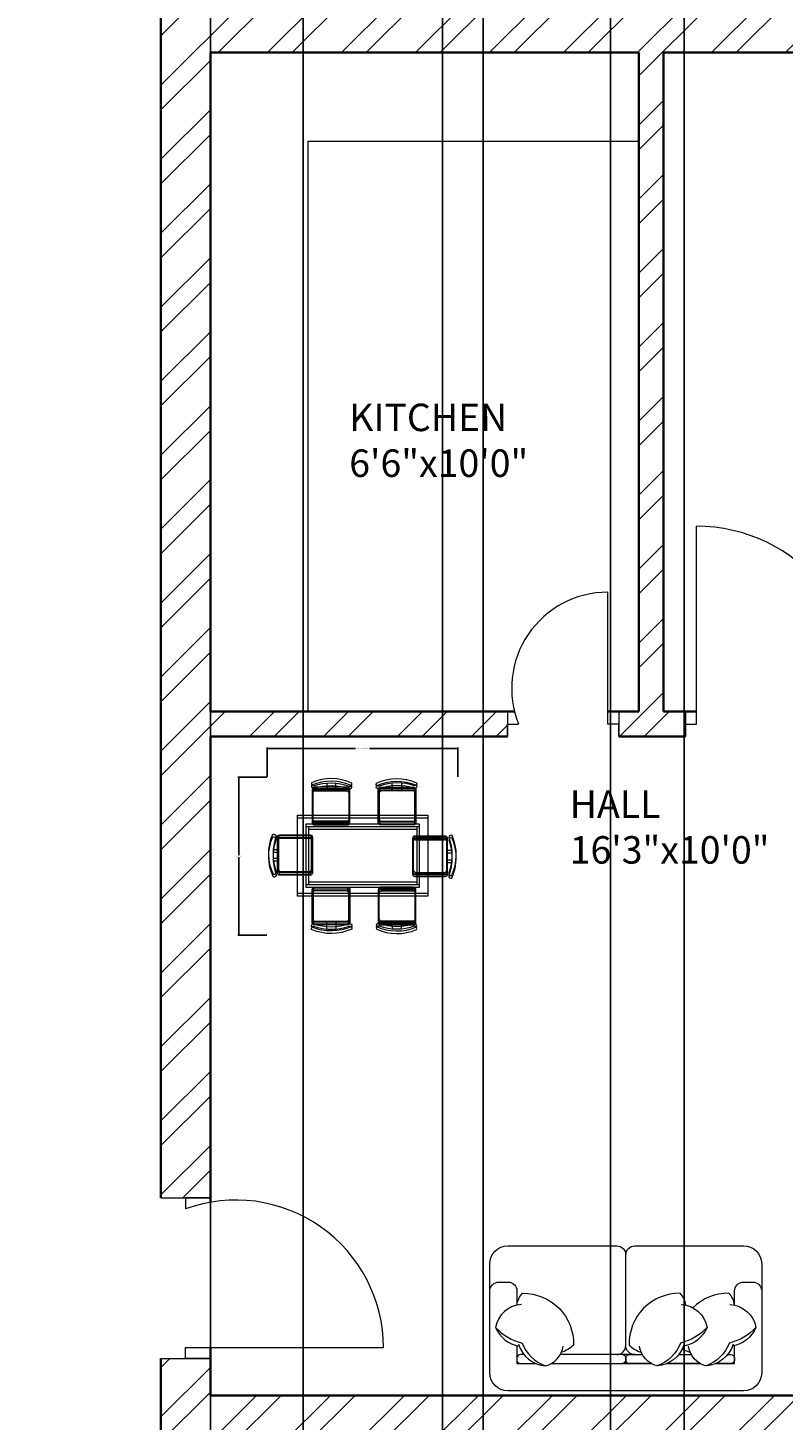
# Model space of a CAD drawing. Units: inches. Extents: x 2552 to 3217, y 1417 to 2737.
# Tile 12 of 25: x 2885 to 3022, y 1885 to 2138. Entities that reach past the tile are written whole.
import ezdxf

# ---------------------------------------------------------------- set-up
doc = ezdxf.new("R2010")
doc.units = ezdxf.units.IN
for name, color, linetype, lineweight in [('A-ANNO-DIMS', 2, 'Continuous', 18), ('A-AREA-IDEN', 7, 'Continuous', 18), ('A-DOOR', 21, 'Continuous', 18), ('A-FLOR-CASE', 9, 'Continuous', 18), ('A-FURN', 8, 'Continuous', 13), ('A-WALL', 7, 'Continuous', 35), ('A-WALL-PATT', 217, 'Continuous', 13)]:
    doc.layers.add(name, color=color, linetype=linetype, lineweight=lineweight)
doc.styles.get("Standard").update_dxf_attribs({"font": 'arial.ttf'})
doc.dimstyles.get("Standard").update_dxf_attribs({"dimtxt": 0.18, "dimasz": 0.18, "dimexe": 0.18, "dimexo": 0.0625, "dimgap": 0.09, "dimtad": 0, "dimtih": 1, "dimtoh": 1, "dimdec": 4, "dimzin": 0, "dimdsep": 46, "dimtxsty": 'Standard', "dimcen": 0.09, "dimadec": 0, "dimazin": 0, "dimtfac": 1, "dimtdec": 4, "dimtofl": 0, "dimtmove": 0, "dimatfit": 3, "dimfxl": 1, "dimtolj": 1, "dimtzin": 0, "dimarcsym": 0})

# ---------------------------------------------------------------- blocks, each defined once
blk = doc.blocks.new('DINING-SET-SIX')
for points in [[(8.15, 26.89, -0.175809), (14.62, 26.84, 0.578392), (15.11, 27.38, 0.214524), (7.8, 27.47, 0.552014), (8.15, 26.89, -0.065079)], [(8.15, 26.89, -0.175809), (14.62, 26.84, 0.578392), (15.11, 27.38, 0.214524), (7.8, 27.47, 0.552014), (8.15, 26.89, -0.065079)], [(20.07, 26.84, -0.578392), (19.58, 27.38, -0.214524), (26.89, 27.47, -0.552014), (26.55, 26.89, 0.175809), (20.07, 26.84)], [(20.07, 26.84, -0.578392), (19.58, 27.38, -0.214524), (26.89, 27.47, -0.552014), (26.55, 26.89, 0.175809), (20.07, 26.84)], [(8.15, 26.41, -0.175809), (14.62, 26.36, 0.578392), (15.11, 26.9, 0.214524), (7.8, 27, 0.552014), (8.15, 26.41, -0.065079)], [(8.15, 26.41, -0.175809), (14.62, 26.36, 0.578392), (15.11, 26.9, 0.214524), (7.8, 27, 0.552014), (8.15, 26.41, -0.065079)], [(14.35, 26.63), (8.33, 26.63, 0.414214), (7.91, 26.21), (7.91, 20.68, 0.414214), (8.33, 20.26), (14.35, 20.26, 0.414214), (14.77, 20.68), (14.77, 26.21, 0.414214), (14.35, 26.63)], [(14.35, 26.63), (8.33, 26.63, 0.414214), (7.91, 26.21), (7.91, 20.68, 0.414214), (8.33, 20.26), (14.35, 20.26, 0.414214), (14.77, 20.68), (14.77, 26.21, 0.414214), (14.35, 26.63)], [(14.35, 26.15), (8.33, 26.15, 0.414214), (7.91, 25.73), (7.91, 20.2, 0.414214), (8.33, 19.78), (14.35, 19.78, 0.414214), (14.77, 20.2), (14.77, 25.73, 0.414214), (14.35, 26.15)], [(14.35, 26.15), (8.33, 26.15, 0.414214), (7.91, 25.73), (7.91, 20.2, 0.414214), (8.33, 19.78), (14.35, 19.78, 0.414214), (14.77, 20.2), (14.77, 25.73, 0.414214), (14.35, 26.15)], [(12.23, 26.63), (12.23, 27.39, -0.064759)], [(12.23, 26.63), (12.23, 27.39, -0.064759)], [(12.23, 26.15), (12.23, 26.91, -0.064759)], [(12.23, 26.15), (12.23, 26.91, -0.064759)], [(20.07, 26.36, -0.578392), (19.58, 26.9, -0.214524), (26.89, 27, -0.552014), (26.55, 26.41, 0.175809), (20.07, 26.36)], [(20.07, 26.36, -0.578392), (19.58, 26.9, -0.214524), (26.89, 27, -0.552014), (26.55, 26.41, 0.175809), (20.07, 26.36)], [(26.36, 26.63, -0.414214), (26.78, 26.21), (26.78, 20.68, -0.414214), (26.36, 20.26), (20.35, 20.26, -0.414214), (19.92, 20.68), (19.92, 26.21, -0.414214), (20.35, 26.63), (26.36, 26.63)], [(26.36, 26.63, -0.414214), (26.78, 26.21), (26.78, 20.68, -0.414214), (26.36, 20.26), (20.35, 20.26, -0.414214), (19.92, 20.68), (19.92, 26.21, -0.414214), (20.35, 26.63), (26.36, 26.63)], [(26.36, 26.15, -0.414214), (26.78, 25.73), (26.78, 20.2, -0.414214), (26.36, 19.78), (20.35, 19.78, -0.414214), (19.92, 20.2), (19.92, 25.73, -0.414214), (20.35, 26.15), (26.36, 26.15)], [(26.36, 26.15, -0.414214), (26.78, 25.73), (26.78, 20.2, -0.414214), (26.36, 19.78), (20.35, 19.78, -0.414214), (19.92, 20.2), (19.92, 25.73, -0.414214), (20.35, 26.15), (26.36, 26.15)], [(22.46, 26.63), (22.46, 27.39, 0.064759)], [(22.46, 26.63), (22.46, 27.39, 0.064759)], [(22.46, 26.15), (22.46, 26.91, 0.064759)], [(22.46, 26.15), (22.46, 26.91, 0.064759)], [(1.37, 11.25, -0.578392), (0.83, 10.76, -0.214524), (0.73, 18.07, -0.552014), (1.32, 17.73, 0.175809), (1.37, 11.25)], [(1.37, 11.25, -0.578392), (0.83, 10.76, -0.214524), (0.73, 18.07, -0.552014), (1.32, 17.73, 0.175809), (1.37, 11.25)], [(1.58, 17.54, -0.414214), (2, 17.96), (7.53, 17.96, -0.414214), (7.95, 17.54), (7.95, 11.53, -0.414214), (7.53, 11.11), (2, 11.11, -0.414214), (1.58, 11.53), (1.58, 17.54)], [(1.58, 17.54, -0.414214), (2, 17.96), (7.53, 17.96, -0.414214), (7.95, 17.54), (7.95, 11.53, -0.414214), (7.53, 11.11), (2, 11.11, -0.414214), (1.58, 11.53), (1.58, 17.54)], [(32.54, 17.33, 0.414214), (32.11, 17.75), (26.59, 17.75, 0.414214), (26.17, 17.33), (26.17, 11.32, 0.414214), (26.59, 10.9), (32.11, 10.9, 0.414214), (32.54, 11.32), (32.54, 17.33)], [(32.54, 17.33, 0.414214), (32.11, 17.75), (26.59, 17.75, 0.414214), (26.17, 17.33), (26.17, 11.32, 0.414214), (26.59, 10.9), (32.11, 10.9, 0.414214), (32.54, 11.32), (32.54, 17.33)], [(32.79, 17.52, -0.175809), (32.75, 11.05, 0.578392), (33.29, 10.56, 0.214524), (33.38, 17.86, 0.552014), (32.79, 17.52, -0.065079)], [(32.79, 17.52, -0.175809), (32.75, 11.05, 0.578392), (33.29, 10.56, 0.214524), (33.38, 17.86, 0.552014), (32.79, 17.52, -0.065079)], [(1.37, 10.78, -0.578392), (0.83, 10.29, -0.214524), (0.73, 17.59, -0.552014), (1.32, 17.25, 0.175809), (1.37, 10.78)], [(1.37, 10.78, -0.578392), (0.83, 10.29, -0.214524), (0.73, 17.59, -0.552014), (1.32, 17.25, 0.175809), (1.37, 10.78)], [(1.58, 17.06, -0.414214), (2, 17.48), (7.53, 17.48, -0.414214), (7.95, 17.06), (7.95, 11.05, -0.414214), (7.53, 10.63), (2, 10.63, -0.414214), (1.58, 11.05), (1.58, 17.06)], [(1.58, 17.06, -0.414214), (2, 17.48), (7.53, 17.48, -0.414214), (7.95, 17.06), (7.95, 11.05, -0.414214), (7.53, 10.63), (2, 10.63, -0.414214), (1.58, 11.05), (1.58, 17.06)], [(32.54, 16.86, 0.414214), (32.11, 17.28), (26.59, 17.28, 0.414214), (26.17, 16.86), (26.17, 10.85, 0.414214), (26.59, 10.42), (32.11, 10.42, 0.414214), (32.54, 10.85), (32.54, 16.86)], [(32.54, 16.86, 0.414214), (32.11, 17.28), (26.59, 17.28, 0.414214), (26.17, 16.86), (26.17, 10.84, 0.414214), (26.59, 10.42), (32.11, 10.42, 0.414214), (32.54, 10.84), (32.54, 16.86)], [(32.79, 17.04, -0.175809), (32.75, 10.57, 0.578392), (33.29, 10.08, 0.214524), (33.38, 17.39, 0.552014), (32.79, 17.04, -0.065079)], [(32.79, 17.04, -0.175809), (32.75, 10.57, 0.578392), (33.29, 10.08, 0.214524), (33.38, 17.39, 0.552014), (32.79, 17.04, -0.065079)], [(1.58, 13.64), (0.82, 13.64, 0.064759)], [(1.58, 13.64), (0.82, 13.64, 0.064759)], [(1.58, 13.16), (0.82, 13.16, 0.064759)], [(1.58, 13.16), (0.82, 13.16, 0.064759)], [(32.54, 13.43), (33.3, 13.43, -0.064759)], [(32.54, 13.43), (33.3, 13.43, -0.064759)], [(32.54, 12.96), (33.3, 12.96, -0.064759)], [(32.54, 12.96), (33.3, 12.96, -0.064759)], [(14.35, 2.06), (8.33, 2.06, -0.414214), (7.91, 2.48), (7.91, 8.01, -0.414214), (8.33, 8.43), (14.35, 8.43, -0.414214), (14.77, 8.01), (14.77, 2.48, -0.414214), (14.35, 2.06)], [(14.35, 2.06), (8.33, 2.06, -0.414214), (7.91, 2.48), (7.91, 8.01, -0.414214), (8.33, 8.43), (14.35, 8.43, -0.414214), (14.77, 8.01), (14.77, 2.48, -0.414214), (14.35, 2.06)], [(14.35, 1.58), (8.33, 1.58, -0.414214), (7.91, 2), (7.91, 7.53, -0.414214), (8.33, 7.95), (14.35, 7.95, -0.414214), (14.77, 7.53), (14.77, 2, -0.414214), (14.35, 1.58)], [(14.35, 1.58), (8.33, 1.58, -0.414214), (7.91, 2), (7.91, 7.53, -0.414214), (8.33, 7.95), (14.35, 7.95, -0.414214), (14.77, 7.53), (14.77, 2, -0.414214), (14.35, 1.58)], [(26.36, 2.06, 0.414214), (26.78, 2.48), (26.78, 8.01, 0.414214), (26.36, 8.43), (20.35, 8.43, 0.414214), (19.92, 8.01), (19.92, 2.48, 0.414214), (20.35, 2.06), (26.36, 2.06)], [(26.36, 2.06, 0.414214), (26.78, 2.48), (26.78, 8.01, 0.414214), (26.36, 8.43), (20.35, 8.43, 0.414214), (19.92, 8.01), (19.92, 2.48, 0.414214), (20.35, 2.06), (26.36, 2.06)], [(26.36, 1.58, 0.414214), (26.78, 2), (26.78, 7.53, 0.414214), (26.36, 7.95), (20.35, 7.95, 0.414214), (19.92, 7.53), (19.92, 2, 0.414214), (20.35, 1.58), (26.36, 1.58)], [(26.36, 1.58, 0.414214), (26.78, 2), (26.78, 7.53, 0.414214), (26.36, 7.95), (20.35, 7.95, 0.414214), (19.92, 7.53), (19.92, 2, 0.414214), (20.35, 1.58), (26.36, 1.58)], [(14.62, 1.85, -0.578392), (15.11, 1.31, -0.214524), (7.8, 1.21, -0.552014), (8.15, 1.8, 0.175809), (14.62, 1.85)], [(14.62, 1.85, -0.578392), (15.11, 1.31, -0.214524), (7.8, 1.21, -0.552014), (8.15, 1.8, 0.175809), (14.62, 1.85)], [(14.62, 1.37, -0.578392), (15.11, 0.83, -0.214524), (7.8, 0.74, -0.552014), (8.15, 1.32, 0.175809), (14.62, 1.37)], [(14.62, 1.37, -0.578392), (15.11, 0.83, -0.214524), (7.8, 0.74, -0.552014), (8.15, 1.32, 0.175809), (14.62, 1.37)], [(12.23, 2.06), (12.23, 1.3, 0.064759)], [(12.23, 2.06), (12.23, 1.3, 0.064759)], [(12.23, 1.58), (12.23, 0.82, 0.064759)], [(12.23, 1.58), (12.23, 0.82, 0.064759)], [(26.55, 1.8, -0.175809), (20.07, 1.85, 0.578392), (19.58, 1.31, 0.214524), (26.89, 1.21, 0.552014), (26.55, 1.8, -0.065079)], [(26.55, 1.8, -0.175809), (20.07, 1.85, 0.578392), (19.58, 1.31, 0.214524), (26.89, 1.21, 0.552014), (26.55, 1.8, -0.065079)], [(26.55, 1.32, -0.175809), (20.07, 1.37, 0.578392), (19.58, 0.83, 0.214524), (26.89, 0.74, 0.552014), (26.55, 1.32, -0.065079)], [(26.55, 1.32, -0.175809), (20.07, 1.37, 0.578392), (19.58, 0.83, 0.214524), (26.89, 0.74, 0.552014), (26.55, 1.32, -0.065079)], [(22.46, 2.06), (22.46, 1.3, -0.064759)], [(22.46, 2.06), (22.46, 1.3, -0.064759)], [(22.46, 1.58), (22.46, 0.82, -0.064759)], [(22.46, 1.58), (22.46, 0.82, -0.064759)]]:
    blk.add_lwpolyline(points, format="xyb")
for points in [[(8.34, 26.44), (14.16, 26.44, -0.414214), (14.58, 26.02), (14.58, 20.87, -0.414214), (14.16, 20.45), (8.34, 20.45, -0.512069), (8.1, 20.87), (8.1, 26.02, -0.512069)], [(8.34, 26.44), (14.16, 26.44, -0.414214), (14.58, 26.02), (14.58, 20.87, -0.414214), (14.16, 20.45), (8.34, 20.45, -0.512069), (8.1, 20.87), (8.1, 26.02, -0.512069)], [(8.34, 25.96), (14.16, 25.96, -0.414214), (14.58, 25.54), (14.58, 20.39, -0.414214), (14.16, 19.97), (8.34, 19.97, -0.512069), (8.1, 20.39), (8.1, 25.54, -0.512069)], [(8.34, 25.96), (14.16, 25.96, -0.414214), (14.58, 25.54), (14.58, 20.39, -0.414214), (14.16, 19.97), (8.34, 19.97, -0.512069), (8.1, 20.39), (8.1, 25.54, -0.512069)], [(26.35, 26.44), (20.53, 26.44, 0.414214), (20.11, 26.02), (20.11, 20.87, 0.414214), (20.53, 20.45), (26.35, 20.45, 0.512069), (26.59, 20.87), (26.59, 26.02, 0.512069)], [(26.35, 26.44), (20.53, 26.44, 0.414214), (20.11, 26.02), (20.11, 20.87, 0.414214), (20.53, 20.45), (26.35, 20.45, 0.512069), (26.59, 20.87), (26.59, 26.02, 0.512069)], [(26.35, 25.96), (20.53, 25.96, 0.414214), (20.11, 25.54), (20.11, 20.39, 0.414214), (20.53, 19.97), (26.35, 19.97, 0.512069), (26.59, 20.39), (26.59, 25.54, 0.512069)], [(26.35, 25.96), (20.53, 25.96, 0.414214), (20.11, 25.54), (20.11, 20.39, 0.414214), (20.53, 19.97), (26.35, 19.97, 0.512069), (26.59, 20.39), (26.59, 25.54, 0.512069)], [(1.77, 17.53), (1.77, 11.72, 0.414214), (2.19, 11.3), (7.34, 11.3, 0.414214), (7.76, 11.72), (7.76, 17.53, 0.512069), (7.34, 17.77), (2.19, 17.77, 0.512069)], [(1.77, 17.53), (1.77, 11.72, 0.414214), (2.19, 11.29), (7.34, 11.29, 0.414214), (7.76, 11.72), (7.76, 17.53, 0.512069), (7.34, 17.77), (2.19, 17.77, 0.512069)], [(1.77, 17.06), (1.77, 11.24, 0.414214), (2.19, 10.82), (7.34, 10.82, 0.414214), (7.76, 11.24), (7.76, 17.06, 0.512069), (7.34, 17.29), (2.19, 17.29, 0.512069)], [(1.77, 17.06), (1.77, 11.24, 0.414214), (2.19, 10.82), (7.34, 10.82, 0.414214), (7.76, 11.24), (7.76, 17.06, 0.512069), (7.34, 17.29), (2.19, 17.29, 0.512069)], [(32.35, 17.33), (32.35, 11.51, -0.414214), (31.93, 11.09), (26.78, 11.09, -0.414214), (26.36, 11.51), (26.36, 17.33, -0.512069), (26.78, 17.56), (31.93, 17.56, -0.512069)], [(32.35, 17.33), (32.35, 11.51, -0.414214), (31.93, 11.09), (26.78, 11.09, -0.414214), (26.36, 11.51), (26.36, 17.33, -0.512069), (26.78, 17.56), (31.93, 17.56, -0.512069)], [(32.35, 16.85), (32.35, 11.03, -0.414214), (31.93, 10.61), (26.78, 10.61, -0.414214), (26.36, 11.03), (26.36, 16.85, -0.512069), (26.78, 17.09), (31.93, 17.09, -0.512069)], [(32.35, 16.85), (32.35, 11.03, -0.414214), (31.93, 10.61), (26.78, 10.61, -0.414214), (26.36, 11.03), (26.36, 16.85, -0.512069), (26.78, 17.09), (31.93, 17.09, -0.512069)], [(8.34, 2.25), (14.16, 2.25, 0.414214), (14.58, 2.67), (14.58, 7.82, 0.414214), (14.16, 8.24), (8.34, 8.24, 0.512069), (8.1, 7.82), (8.1, 2.67, 0.512069)], [(8.34, 2.25), (14.16, 2.25, 0.414214), (14.58, 2.67), (14.58, 7.82, 0.414214), (14.16, 8.24), (8.34, 8.24, 0.512069), (8.1, 7.82), (8.1, 2.67, 0.512069)], [(8.34, 1.77), (14.16, 1.77, 0.414214), (14.58, 2.19), (14.58, 7.34, 0.414214), (14.16, 7.76), (8.34, 7.76, 0.512069), (8.1, 7.34), (8.1, 2.19, 0.512069)], [(8.34, 1.77), (14.16, 1.77, 0.414214), (14.58, 2.19), (14.58, 7.34, 0.414214), (14.16, 7.76), (8.34, 7.76, 0.512069), (8.1, 7.34), (8.1, 2.19, 0.512069)], [(26.35, 2.25), (20.53, 2.25, -0.414214), (20.11, 2.67), (20.11, 7.82, -0.414214), (20.53, 8.24), (26.35, 8.24, -0.512069), (26.59, 7.82), (26.59, 2.67, -0.512069)], [(26.35, 2.25), (20.53, 2.25, -0.414214), (20.11, 2.67), (20.11, 7.82, -0.414214), (20.53, 8.24), (26.35, 8.24, -0.512069), (26.59, 7.82), (26.59, 2.67, -0.512069)], [(26.35, 1.77), (20.53, 1.77, -0.414214), (20.11, 2.19), (20.11, 7.34, -0.414214), (20.53, 7.76), (26.35, 7.76, -0.512069), (26.59, 7.34), (26.59, 2.19, -0.512069)], [(26.35, 1.77), (20.53, 1.77, -0.414214), (20.11, 2.19), (20.11, 7.34, -0.414214), (20.53, 7.76), (26.35, 7.76, -0.512069), (26.59, 7.34), (26.59, 2.19, -0.512069)]]:
    blk.add_lwpolyline(points, format="xyb", close=True)
for points in [[(10.55, 27.4), (10.55, 26.63)], [(10.55, 27.4), (10.55, 26.63)], [(10.55, 26.93), (10.55, 26.15)], [(10.55, 26.92), (10.55, 26.15)], [(24.14, 27.4), (24.14, 26.63)], [(24.14, 27.4), (24.14, 26.63)], [(24.14, 26.93), (24.14, 26.15)], [(24.14, 26.92), (24.14, 26.15)], [(0.81, 15.32), (1.58, 15.32)], [(0.81, 15.32), (1.58, 15.32)], [(0.81, 14.84), (1.58, 14.84)], [(0.81, 14.84), (1.58, 14.84)], [(33.31, 15.11), (32.54, 15.11)], [(33.31, 15.11), (32.54, 15.11)], [(33.31, 14.64), (32.54, 14.64)], [(33.31, 14.64), (32.54, 14.64)], [(10.55, 1.29), (10.55, 2.06)], [(10.55, 1.28), (10.55, 2.06)], [(10.55, 0.81), (10.55, 1.58)], [(10.55, 0.81), (10.55, 1.58)], [(24.14, 1.29), (24.14, 2.06)], [(24.14, 1.28), (24.14, 2.06)], [(24.14, 0.81), (24.14, 1.58)], [(24.14, 0.81), (24.14, 1.58)]]:
    blk.add_lwpolyline(points)
for points in [[(5.21, 21.55), (28.98, 21.55), (28.98, 7.29), (5.21, 7.29)], [(5.21, 21.55), (28.98, 21.55), (28.98, 7.29), (5.21, 7.29)], [(5.21, 21.08), (28.98, 21.08), (28.98, 6.81), (5.21, 6.81)], [(5.21, 21.07), (28.98, 21.07), (28.98, 6.81), (5.21, 6.81)], [(6.79, 19.97), (27.39, 19.97), (27.39, 8.87), (6.79, 8.87)], [(6.79, 19.97), (27.39, 19.97), (27.39, 8.87), (6.79, 8.87)], [(6.79, 19.49), (27.39, 19.49), (27.39, 8.4), (6.79, 8.4)], [(6.79, 19.49), (27.39, 19.49), (27.39, 8.4), (6.79, 8.4)], [(7.27, 19.49), (26.92, 19.49), (26.92, 9.35), (7.27, 9.35)], [(7.27, 19.49), (26.92, 19.49), (26.92, 9.35), (7.27, 9.35)], [(7.27, 19.01), (26.92, 19.01), (26.92, 8.87), (7.27, 8.87)], [(7.27, 19.01), (26.92, 19.01), (26.92, 8.87), (7.27, 8.87)]]:
    blk.add_lwpolyline(points, close=True)
blk = doc.blocks.new('*D31')
at = {"layer": 'A-ANNO-DIMS', "color": 0, "lineweight": -2, "transparency": 16777216}
for p, q in [((2928.21, 2001.66), (2928.21, 2006.97)), ((2928.39, 2006.79), (2944.27, 2006.79)), ((2962.7, 2006.79), (2946.82, 2006.79)), ((2962.88, 2001.66), (2962.88, 2006.97))]:
    blk.add_line(p, q, dxfattribs=at)
at = {"layer": 'A-ANNO-DIMS', "color": 0, "transparency": 16777216}
for points in [[(2928.39, 2006.82), (2928.39, 2006.76), (2928.21, 2006.79)], [(2962.7, 2006.82), (2962.7, 2006.76), (2962.88, 2006.79)]]:
    blk.add_solid(points, dxfattribs=at)
at = {"layer": 'Defpoints', "color": 0, "transparency": 16777216}
for p in [(2962.88, 2006.79), (2928.21, 2001.59), (2962.88, 2001.59)]:
    blk.add_point(p, dxfattribs=at)
at = {"layer": 'A-ANNO-DIMS', "color": 0, "transparency": 16777216, "insert": (2945.55, 2006.79), "char_height": 0.18, "attachment_point": 5}
blk.add_mtext('\\A1;DINING SET 35 TYP.', dxfattribs=at)
blk = doc.blocks.new('*D32')
at = {"layer": 'A-ANNO-DIMS', "color": 0, "lineweight": -2, "transparency": 16777216}
for p, q in [((2928.15, 2001.59), (2922.83, 2001.59)), ((2923.01, 2001.41), (2923.01, 1987.39)), ((2923.01, 1973.01), (2923.01, 1987.03)), ((2928.15, 1972.83), (2922.83, 1972.83))]:
    blk.add_line(p, q, dxfattribs=at)
at = {"layer": 'A-ANNO-DIMS', "color": 0, "transparency": 16777216}
for points in [[(2922.98, 2001.41), (2923.04, 2001.41), (2923.01, 2001.59)], [(2922.98, 1973.01), (2923.04, 1973.01), (2923.01, 1972.83)]]:
    blk.add_solid(points, dxfattribs=at)
at = {"layer": 'Defpoints', "color": 0, "transparency": 16777216}
for p in [(2923.01, 2001.59), (2928.21, 2001.59), (2928.21, 1972.83)]:
    blk.add_point(p, dxfattribs=at)
at = {"layer": 'A-ANNO-DIMS', "color": 0, "transparency": 16777216, "insert": (2923.01, 1987.21), "char_height": 0.18, "attachment_point": 5}
blk.add_mtext('\\A1;29 TYP.', dxfattribs=at)
blk = doc.blocks.new('*D56')
at = {"layer": 'A-ANNO-DIMS', "color": 0, "lineweight": -2, "transparency": 16777216}
for p, q in [((2967.49, 2515.95), (2967.49, 1482.53)), ((2990.69, 2515.95), (2990.69, 1482.53)), ((2967.67, 1482.71), (2978.76, 1482.71)), ((2990.51, 1482.71), (2979.41, 1482.71))]:
    blk.add_line(p, q, dxfattribs=at)
at = {"layer": 'A-ANNO-DIMS', "color": 0, "transparency": 16777216}
for points in [[(2967.67, 1482.74), (2967.67, 1482.68), (2967.49, 1482.71)], [(2990.51, 1482.74), (2990.51, 1482.68), (2990.69, 1482.71)]]:
    blk.add_solid(points, dxfattribs=at)
at = {"layer": 'Defpoints', "color": 0, "transparency": 16777216}
for p in [(2967.49, 2516.01), (2990.69, 2516.01), (2990.69, 1482.71)]:
    blk.add_point(p, dxfattribs=at)
at = {"layer": 'A-ANNO-DIMS', "color": 0, "transparency": 16777216, "insert": (2979.09, 1482.71), "char_height": 0.18, "attachment_point": 5}
blk.add_mtext('\\A1;23.2', dxfattribs=at)
blk = doc.blocks.new('*D57')
at = {"layer": 'A-ANNO-DIMS', "color": 0, "lineweight": -2, "transparency": 16777216}
for p, q in [((3004.08, 2515.95), (3004.08, 1482.53)), ((3036.34, 2515.95), (3036.34, 1482.53)), ((3004.26, 1482.71), (3019.75, 1482.71)), ((3036.16, 1482.71), (3020.68, 1482.71))]:
    blk.add_line(p, q, dxfattribs=at)
at = {"layer": 'A-ANNO-DIMS', "color": 0, "transparency": 16777216}
for points in [[(3004.26, 1482.74), (3004.26, 1482.68), (3004.08, 1482.71)], [(3036.16, 1482.74), (3036.16, 1482.68), (3036.34, 1482.71)]]:
    blk.add_solid(points, dxfattribs=at)
at = {"layer": 'Defpoints', "color": 0, "transparency": 16777216}
for p in [(3004.08, 2516.01), (3036.34, 2516.01), (3036.34, 1482.71)]:
    blk.add_point(p, dxfattribs=at)
at = {"layer": 'A-ANNO-DIMS', "color": 0, "transparency": 16777216, "insert": (3020.21, 1482.71), "char_height": 0.18, "attachment_point": 5}
blk.add_mtext('\\A1;32.255', dxfattribs=at)
blk = doc.blocks.new('*D64')
at = {"layer": 'A-ANNO-DIMS', "color": 0, "lineweight": -2, "transparency": 16777216}
for p, q in [((2646.35, 1551.58), (2646.35, 2709.49)), ((2646.53, 2709.31), (2802.77, 2709.31)), ((2959.93, 2709.31), (2803.69, 2709.31)), ((2960.11, 1551.58), (2960.11, 2709.49))]:
    blk.add_line(p, q, dxfattribs=at)
at = {"layer": 'A-ANNO-DIMS', "color": 0, "transparency": 16777216}
for points in [[(2646.53, 2709.34), (2646.53, 2709.28), (2646.35, 2709.31)], [(2959.93, 2709.34), (2959.93, 2709.28), (2960.11, 2709.31)]]:
    blk.add_solid(points, dxfattribs=at)
at = {"layer": 'Defpoints', "color": 0, "transparency": 16777216}
for p in [(2960.11, 2709.31), (2646.35, 1551.51), (2960.11, 1551.51)]:
    blk.add_point(p, dxfattribs=at)
at = {"layer": 'A-ANNO-DIMS', "color": 0, "transparency": 16777216, "insert": (2803.23, 2709.31), "char_height": 0.18, "attachment_point": 5}
blk.add_mtext('\\A1;313.76', dxfattribs=at)
blk = doc.blocks.new('*D67')
at = {"layer": 'A-ANNO-DIMS', "color": 0, "lineweight": -2, "transparency": 16777216}
for p, q in [((2917.85, 2640.45), (2917.85, 1482.53)), ((2934.77, 2624.73), (2934.77, 1482.53)), ((2918.03, 1482.71), (2925.86, 1482.71)), ((2934.59, 1482.71), (2926.76, 1482.71))]:
    blk.add_line(p, q, dxfattribs=at)
at = {"layer": 'A-ANNO-DIMS', "color": 0, "transparency": 16777216}
for points in [[(2918.03, 1482.74), (2918.03, 1482.68), (2917.85, 1482.71)], [(2934.59, 1482.74), (2934.59, 1482.68), (2934.77, 1482.71)]]:
    blk.add_solid(points, dxfattribs=at)
at = {"layer": 'Defpoints', "color": 0, "transparency": 16777216}
for p in [(2917.85, 2640.51), (2934.77, 2624.79), (2934.77, 1482.71)]:
    blk.add_point(p, dxfattribs=at)
at = {"layer": 'A-ANNO-DIMS', "color": 0, "transparency": 16777216, "insert": (2926.31, 1482.71), "char_height": 0.18, "attachment_point": 5}
blk.add_mtext('\\A1;16.912', dxfattribs=at)

msp = doc.modelspace()

# ---------------------------------------------------------------- hatches: boundary and pattern name
at = {"layer": 'A-WALL-PATT'}
h = msp.add_hatch(dxfattribs=at)
h.set_pattern_fill('ANSI32', color=256)
h.paths.add_polyline_path([(2756.676, 2649.5125), (2637.3535, 2649.5125), (2637.3535, 2617.9626), (2641.8535, 2617.9626), (2646.3535, 2617.9626), (2646.3535, 2640.5125), (2724.3535, 2640.5125), (2724.3535, 2520.5125), (2720.299, 2520.5125), (2720.299, 2516.0125), (2733.4075, 2516.0125), (2733.4075, 2518.2213), (2733.4075, 2520.5125), (2728.8535, 2520.5125), (2728.8535, 2640.5125), (2756.676, 2640.5125)])
h.paths.add_polyline_path([(2848.8535, 2649.5125), (2804.676, 2649.5125), (2804.676, 2640.5125), (2839.8535, 2640.5125), (2839.8535, 2598.3517), (2848.8535, 2598.3517)])
h.paths.add_polyline_path([(2646.3535, 2516.0125), (2697.9593, 2516.0125), (2697.9593, 2518.2625), (2697.9593, 2520.5125), (2646.3535, 2520.5125), (2646.3535, 2581.9626), (2637.3535, 2581.9626), (2637.3535, 2364.3298), (2646.3535, 2364.3298), (2646.3535, 2387.0125), (2724.3535, 2387.0125), (2724.3535, 2267.0125), (2721.0443, 2267.0125), (2721.0443, 2262.5125), (2733.7854, 2262.5125), (2733.7854, 2264.7625), (2733.7854, 2267.0125), (2728.8535, 2267.0125), (2728.8535, 2387.0125), (2839.8535, 2387.0125), (2839.8535, 2363.8387), (2848.8535, 2363.8387), (2848.8535, 2403.7415), (2844.3535, 2403.7415), (2839.8535, 2403.7415), (2839.8535, 2396.0125), (2646.3535, 2396.0125)])
h.paths.add_polyline_path([(2848.8535, 2550.3517), (2844.3535, 2550.3517), (2839.8535, 2550.3517), (2839.8535, 2520.5125), (2801.9195, 2520.5125), (2801.9195, 2518.2625), (2801.9195, 2516.0125), (2839.8535, 2516.0125), (2839.8535, 2507.5813), (2848.8535, 2507.5813)], flags=17)
h.paths.add_polyline_path([(2848.8535, 2483.5813), (2844.3535, 2483.5813), (2839.8535, 2483.5813), (2839.8535, 2468.0125), (2773.8535, 2468.0125), (2773.8535, 2516.0125), (2778.1336, 2516.0125), (2778.1336, 2520.5125), (2766.696, 2520.5125), (2766.696, 2518.2625), (2766.696, 2516.0125), (2769.3535, 2516.0125), (2769.3535, 2463.5125), (2839.8535, 2463.5125), (2839.8535, 2431.0782), (2848.8535, 2431.0782)], flags=17)
h.paths.add_polyline_path([(2917.8535, 2569.2764), (2913.3535, 2569.2764), (2908.8535, 2569.2764), (2908.8535, 2433.001), (2917.8535, 2433.001), (2917.8535, 2516.0125), (2967.486, 2516.0125), (2967.486, 2520.5125), (2917.8535, 2520.5125)])
h.paths.add_polyline_path([(3000.3535, 2640.5125), (2995.8535, 2640.5125), (2995.8535, 2520.5125), (2990.688, 2520.5125), (2990.688, 2516.0125), (3004.0844, 2516.0125), (3004.0844, 2518.2625), (3004.0844, 2520.5125), (3000.3535, 2520.5125)])
h.paths.add_polyline_path([(3120.3535, 2561.3689), (3115.8535, 2561.3689), (3111.3535, 2561.3689), (3111.3535, 2520.5125), (3070.9814, 2520.5125), (3070.9814, 2518.2625), (3070.9814, 2516.0125), (3111.3535, 2516.0125), (3111.3535, 2505.1841), (3120.3535, 2505.1841)])
h.paths.add_polyline_path([(3120.3535, 2481.1841), (3115.8535, 2481.1841), (3111.3535, 2481.1841), (3111.3535, 2468.0125), (3045.3535, 2468.0125), (3045.3535, 2516.0125), (3048.9787, 2516.0125), (3048.9787, 2520.5125), (3036.3395, 2520.5125), (3036.3395, 2516.0125), (3040.8535, 2516.0125), (3040.8535, 2463.5125), (3111.3535, 2463.5125), (3111.3535, 2396.0125), (2917.8535, 2396.0125), (2917.8535, 2403.4124), (2913.3535, 2403.4124), (2908.8535, 2403.4124), (2908.8535, 2182.5756), (2917.8535, 2182.5756), (2917.8535, 2262.5125), (2968.001, 2262.5125), (2968.001, 2264.7625), (2968.001, 2267.0125), (2917.8535, 2267.0125), (2917.8535, 2387.0125), (3111.3535, 2387.0125), (3111.3535, 2352.2435), (3120.3535, 2352.2435)])
h.paths.add_polyline_path([(3120.3535, 2304.2435), (3115.8535, 2304.2435), (3111.3535, 2304.2435), (3111.3535, 2267.0125), (3073.8616, 2267.0125), (3073.8616, 2264.7625), (3073.8616, 2262.5125), (3111.3535, 2262.5125), (3111.3535, 2252.376), (3120.3535, 2252.376)], flags=17)
h.paths.add_polyline_path([(3120.3535, 2228.376), (3115.8535, 2228.376), (3111.3535, 2228.376), (3111.3535, 2214.5125), (3045.3535, 2214.5125), (3045.3535, 2262.5125), (3049.3096, 2262.5125), (3049.3096, 2267.0125), (3035.0125, 2267.0125), (3035.0125, 2262.5125), (3040.8535, 2262.5125), (3040.8535, 2210.0125), (3111.3535, 2210.0125), (3111.3535, 2142.5125), (2917.8535, 2142.5125), (2917.8535, 2150.2408), (2913.3535, 2150.2408), (2908.8535, 2150.2408), (2908.8535, 1924.9905), (2917.8535, 1924.9905), (2917.8535, 2009.0125), (2971.959, 2009.0125), (2971.959, 2011.2625), (2971.959, 2013.5125), (2917.8535, 2013.5125), (2917.8535, 2133.5125), (2995.8535, 2133.5125), (2995.8535, 2013.5125), (2992.1797, 2013.5125), (2992.1797, 2009.0125), (3004.3344, 2009.0125), (3004.3344, 2011.2625), (3004.3344, 2013.5125), (3000.3535, 2013.5125), (3000.3535, 2133.5125), (3111.3535, 2133.5125), (3111.3535, 2115.0291), (3120.3535, 2115.0291)])
h.paths.add_polyline_path([(3000.3535, 2387.0125), (2995.8535, 2387.0125), (2995.8535, 2267.0125), (2991.3326, 2267.0125), (2991.3326, 2262.5125), (3004.1044, 2262.5125), (3004.1044, 2264.7625), (3004.1044, 2267.0125), (3000.3535, 2267.0125)], flags=17)
h.paths.add_polyline_path([(3120.3535, 1973.2388), (3115.8535, 1973.2388), (3111.3535, 1973.2388), (3111.3535, 1961.0125), (3045.3535, 1961.0125), (3045.3535, 2009.0125), (3048.9101, 2009.0125), (3048.9101, 2013.5125), (3037.105, 2013.5125), (3037.105, 2011.2625), (3037.105, 2009.0125), (3040.8535, 2009.0125), (3040.8535, 1956.5125), (3111.3535, 1956.5125), (3111.3535, 1889.0125), (2917.8535, 1889.0125), (2917.8535, 1895.7215), (2913.3535, 1895.7215), (2908.8535, 1895.7215), (2908.8535, 1844.2217), (2917.8535, 1844.2217), (2917.8535, 1880.0125), (3111.3535, 1880.0125), (3111.3535, 1846.9541), (3120.3535, 1846.9541)])
h.paths.add_polyline_path([(3120.3535, 2067.0291), (3111.3535, 2067.0291), (3111.3535, 2013.5125), (3071.3001, 2013.5125), (3071.3001, 2009.0125), (3111.3535, 2009.0125), (3111.3535, 1997.2388), (3120.3535, 1997.2388)], flags=0)
h.paths.add_polyline_path([(3120.3535, 1798.9541), (3115.8535, 1798.9541), (3111.3535, 1798.9541), (3111.3535, 1760.0125), (3071.2497, 1760.0125), (3071.2497, 1757.7625), (3071.2497, 1755.5125), (3111.3535, 1755.5125), (3111.3535, 1746.162), (3120.3535, 1746.2478)])
h.paths.add_polyline_path([(3120.3535, 1722.2049), (3111.3535, 1722.2049), (3111.3535, 1707.5125), (3045.3535, 1707.5125), (3045.3535, 1755.5125), (3048.6624, 1755.5125), (3048.6624, 1760.0125), (3035.3703, 1760.0125), (3035.3703, 1755.5125), (3040.8535, 1755.5125), (3040.8535, 1703.0125), (3111.3535, 1703.0125), (3111.3535, 1635.5125), (2917.8535, 1635.5125), (2917.8535, 1643.1366), (2913.3535, 1643.1366), (2908.8535, 1643.1366), (2908.8535, 1626.5125), (3120.3535, 1626.5125)])
h.paths.add_polyline_path([(2917.8535, 1755.5125), (2973.2287, 1755.5125), (2973.2287, 1757.7625), (2973.2287, 1760.0125), (2917.8535, 1760.0125), (2917.8535, 1808.2217), (2913.3535, 1808.2217), (2908.8535, 1808.2217), (2908.8535, 1676.1665), (2917.8535, 1676.1665)])
h.paths.add_polyline_path([(3000.3535, 1880.0125), (2995.8535, 1880.0125), (2995.8535, 1760.0125), (2992.9329, 1760.0125), (2992.9329, 1755.5125), (3003.8766, 1755.5125), (3003.8766, 1757.7625), (3003.8766, 1760.0125), (3000.3535, 1760.0125)])
h.paths.add_polyline_path([(2848.8535, 1896.6971), (2844.3535, 1896.6971), (2839.8535, 1896.6971), (2839.8535, 1889.0125), (2646.3535, 1889.0125), (2646.3535, 2009.0125), (2700.5253, 2009.0125), (2700.5253, 2011.2625), (2700.5253, 2013.5125), (2646.3535, 2013.5125), (2646.3535, 2053.1812), (2641.8535, 2053.1812), (2637.3535, 2053.1812), (2637.3535, 1836.254), (2646.3535, 1836.254), (2646.3535, 1880.0125), (2724.3535, 1880.0125), (2724.3535, 1760.0125), (2721.2473, 1760.0125), (2721.2473, 1755.5125), (2731.9187, 1755.5125), (2731.9187, 1757.7625), (2731.9187, 1760.0125), (2728.8535, 1760.0125), (2728.8535, 1880.0125), (2839.8535, 1880.0125), (2839.8535, 1840.3813), (2848.8535, 1840.3813)])
h.paths.add_polyline_path([(2848.8535, 1792.3813), (2844.3535, 1792.3813), (2839.8535, 1792.3813), (2839.8535, 1760.0125), (2797.8845, 1760.0125), (2797.8845, 1755.5125), (2839.8535, 1755.5125), (2839.8535, 1743.3688), (2844.3535, 1743.3688), (2848.8535, 1743.3688)], flags=0)
h.paths.add_polyline_path([(2848.8535, 1719.3688), (2844.3535, 1719.3688), (2839.8535, 1719.3688), (2839.8535, 1707.5125), (2773.8535, 1707.5125), (2773.8535, 1755.5125), (2777.716, 1755.5125), (2777.716, 1760.0125), (2760.9247, 1760.0125), (2760.9247, 1757.9721), (2760.9247, 1755.5125), (2769.3535, 1755.5125), (2769.3535, 1703.0125), (2839.8535, 1703.0125), (2839.8535, 1673.0277), (2848.8535, 1672.9407)], flags=0)
h.paths.add_polyline_path([(2646.3535, 1755.5125), (2702.9171, 1755.5125), (2702.9171, 1757.7625), (2702.9171, 1760.0125), (2646.3535, 1760.0125), (2646.3535, 1800.254), (2641.8535, 1800.254), (2637.3535, 1800.254), (2637.3535, 1626.5125), (2848.8535, 1626.5125), (2848.8535, 1643.1187), (2844.3535, 1643.1187), (2839.8535, 1643.1187), (2839.8535, 1635.5125), (2646.3535, 1635.5125)])
h.paths.add_polyline_path([(2848.8535, 2148.8427), (2844.3535, 2148.8427), (2839.8535, 2148.8427), (2839.8535, 2142.5125), (2646.3535, 2142.5125), (2646.3535, 2262.5125), (2701.3562, 2262.5125), (2701.3562, 2264.7625), (2701.3562, 2267.0125), (2646.3535, 2267.0125), (2646.3535, 2328.3298), (2637.3535, 2328.3298), (2637.3535, 2089.1812), (2646.3535, 2089.1812), (2646.3535, 2133.5125), (2839.8535, 2133.5125), (2839.8535, 2097.5966), (2848.8535, 2097.5966)])
h.paths.add_polyline_path([(2728.8535, 2133.5125), (2724.3535, 2133.5125), (2724.3535, 2013.5125), (2719.6039, 2013.5125), (2719.6039, 2009.0125), (2732.5784, 2009.0125), (2732.5784, 2011.2625), (2732.5784, 2013.5125), (2728.8535, 2013.5125)])
h.paths.add_polyline_path([(2848.8535, 1970.0557), (2844.3535, 1970.0557), (2839.8535, 1970.0557), (2839.8535, 1961.0125), (2773.8535, 1961.0125), (2773.8535, 2009.0125), (2777.3388, 2009.0125), (2777.3388, 2013.5125), (2764.7681, 2013.5125), (2764.7681, 2009.0125), (2769.3535, 2009.0125), (2769.3535, 1956.5125), (2839.8535, 1956.5125), (2839.8535, 1924.7199), (2848.8535, 1924.7199)], flags=17)
h.paths.add_polyline_path([(2848.8535, 2049.5966), (2844.3535, 2049.5966), (2839.8535, 2049.5966), (2839.8535, 2013.5125), (2798.198, 2013.5125), (2798.198, 2011.2625), (2798.198, 2009.0125), (2839.8535, 2009.0125), (2839.8535, 1994.0557), (2848.8535, 1994.0557)], flags=17)
h.paths.add_polyline_path([(2848.8535, 2315.8387), (2839.8535, 2315.8387), (2839.8535, 2267.0125), (2799.3375, 2267.0125), (2799.3375, 2264.7625), (2799.3375, 2262.5125), (2839.8535, 2262.5125), (2839.8535, 2253.2843), (2848.8535, 2253.2843)], flags=17)
h.paths.add_polyline_path([(2848.8535, 2229.2843), (2839.8535, 2229.2843), (2839.8535, 2177.6936), (2848.8535, 2177.6936)], flags=17)
h.paths.add_polyline_path([(2839.8535, 2214.5125), (2773.8535, 2214.5125), (2773.8535, 2262.5125), (2777.6984, 2262.5125), (2777.6984, 2267.0125), (2763.8226, 2267.0125), (2763.8226, 2262.5125), (2769.3535, 2262.5125), (2769.3535, 2210.0125), (2839.8535, 2210.0125)], flags=17)
h.paths.add_polyline_path([(3050.32, 2520.2817), (3088.9114, 2520.2817), (3088.9114, 2538.939), (3050.32, 2538.939)], flags=9)

# ---------------------------------------------------------------- linework, layer by layer
at = {"layer": 'A-DOOR'}
for p, q in [((3006.3344, 2011.2625), (3006.3344, 2047.2625)), ((2990.1797, 2011.2625), (2990.1797, 2035.2625)), ((2971.959, 2013.5125), (2971.959, 2009.0125)), ((2992.1797, 2013.5125), (2992.1797, 2009.0125)), ((3004.3344, 2013.5125), (3004.3344, 2009.0125)), ((2971.959, 2009.0125), (2971.959, 2011.2625)), ((2971.959, 2011.2625), (2973.959, 2011.2625)), ((2992.1797, 2011.2625), (2990.1797, 2011.2625)), ((2992.1797, 2009.0125), (2992.1797, 2011.2625)), ((3004.3344, 2009.0125), (3004.3344, 2011.2625)), ((3004.3344, 2011.2625), (3006.3344, 2011.2625)), ((2908.8535, 1924.9905), (2917.8535, 1924.9905)), ((2917.8535, 1924.9905), (2913.3535, 1924.9905)), ((2913.3535, 1924.9905), (2913.3535, 1922.9905)), ((2913.3535, 1895.7215), (2913.3535, 1897.7215)), ((2913.3535, 1897.7215), (2949.3535, 1897.7215)), ((2908.8535, 1895.7215), (2917.8535, 1895.7215)), ((2917.8535, 1895.7215), (2913.3535, 1895.7215)), ((2913.3535, 1895.7215), (2913.3535, 1895.7215))]:
    msp.add_line(p, q, dxfattribs=at)
for centre, radius, start, end in [((3006.3344, 2017.766), 29.4965, 347.262555, 90), ((2990.1797, 2017.7811), 17.4814, 90, 201.893601), ((2922.4852, 1897.7215), 26.8683, 0, 109.868866)]:
    msp.add_arc(centre, radius, start, end, dxfattribs=at)
at = {"layer": 'A-FLOR-CASE'}
for p, q in [((2935.6487, 2013.5125), (2935.6487, 2117.3875)), ((2935.6487, 2117.3875), (2995.8535, 2117.3875))]:
    msp.add_line(p, q, dxfattribs=at)
at = {"layer": 'A-FURN', "ltscale": 0.03}
msp.add_lwpolyline([(2991.8115, 1916.2491, -0.41421356), (2993.4611, 1914.5995, -0.41421356), (2995.1106, 1916.2491), (3014.9054, 1916.2491, -0.41421356), (3018.2045, 1912.9499), (3018.2045, 1893.1552, -0.41421356), (3014.9054, 1889.856), (2972.0168, 1889.856, -0.41421356), (2968.7176, 1893.1552), (2968.7176, 1912.9499, -0.41421356), (2972.0168, 1916.2491), (2991.8115, 1916.2491, -0.41421356), (2993.4611, 1914.5995, -0.41421356), (2995.1106, 1916.2491)], format="xyb", dxfattribs=at)
at = {"layer": 'A-FURN'}
for points in [[(2991.8115, 1896.4543, 0.41421356), (2993.4611, 1898.1039), (2993.4611, 1914.5995, 0.41421356)], [(2995.1106, 1896.4543, -0.41421356), (2993.4611, 1898.1039), (2993.4611, 1914.5995, -0.41421356)], [(2968.7176, 1908.0012, -0.41421356), (2970.3672, 1909.6508), (2972.0168, 1909.6508, -0.41421356), (2973.6663, 1908.0012), (2973.6663, 1905.4455)], [(3013.2558, 1905.4455), (3013.2558, 1908.0012, -0.41421356), (3014.9054, 1909.6508), (3016.555, 1909.6508, -0.41421356), (3018.2045, 1908.0012)], [(2973.6627, 1905.4447, -0.16554063), (2974.6832, 1907.6242, -0.42598917), (2983.9475, 1898.1744, -0.12152332), (2981.7483, 1896.872, 7.11546429)], [(3004.3733, 1905.4447, 0.16554063), (3003.3528, 1907.6242, 0.42598917), (2994.0886, 1898.1744, 0.12152332), (2996.2877, 1896.872, -7.11546429)], [(3013.2594, 1905.4447, 0.16554063), (3012.239, 1907.6242, 0.20023115), (3005.6908, 1904.9698, 0.12152332)], [(2974.4941, 1905.5453, 0.35677236), (2969.7675, 1901.3874, 0.24954205), (2974.0503, 1897.9609, -9.61688035)], [(3003.5419, 1905.5453, -0.35677236), (3008.2686, 1901.3874, -0.24954205), (3003.9858, 1897.9609, 9.61688035)], [(3012.428, 1905.5453, -0.35677236), (3017.1547, 1901.3874, -0.24954205), (3012.8719, 1897.9609, 9.61688035)], [(2969.7675, 1901.3874, 0.14772988), (2974.5887, 1898.5524, 0.21334276), (2978.8427, 1894.3945, 0.17866181)], [(3008.2686, 1901.3874, -0.14772988), (3003.4474, 1898.5524, -0.21334276), (2999.1934, 1894.3945, -0.17866181)], [(3017.1547, 1901.3874, -0.14772988), (3012.3335, 1898.5524, -0.21334276), (3008.0795, 1894.3945, -0.17866181)], [(2974.9251, 1896.4543), (2974.3261, 1896.4543, 0.41421356), (2973.6663, 1895.7945), (2973.6663, 1895.4646, 0.41421356), (2974.3261, 1894.8047)], [(2973.9226, 1898.3265, 0.30666349), (2978.8427, 1894.3945, 0.30632997), (2982.0568, 1897.9854, -0.87284716)], [(2979.8808, 1894.8047), (2992.8013, 1894.8047, 0.41421356), (2993.4611, 1895.4646), (2993.4611, 1895.7945, 0.41421356), (2992.8013, 1896.4543), (2981.5418, 1896.4543, 0.41421356)], [(2991.8115, 1896.4543, 0.41421356), (2993.4611, 1898.1039)], [(2995.1106, 1896.4543, -0.41421356), (2993.4611, 1898.1039)], [(2998.1552, 1894.8047), (2994.1209, 1894.8047, -0.41421356), (2993.4611, 1895.4646), (2993.4611, 1895.7945, -0.41421356), (2994.1209, 1896.4543), (2996.4942, 1896.4543, -0.41421356)], [(3004.1134, 1898.3265, -0.30666349), (2999.1934, 1894.3945, -0.30632997), (2995.9792, 1897.9854, 0.87284716)], [(3003.1109, 1896.4543), (3005.3803, 1896.4543, -0.41421356)], [(3003.7909, 1897.5169, 0.07186538), (3005.1738, 1896.872, -7.11546429)], [(3012.9995, 1898.3265, -0.30666349), (3008.0795, 1894.3945, -0.30632997), (3004.8654, 1897.9854, 0.87284716)], [(3009.7856, 1894.8047), (3013.2558, 1894.8047), (3013.2558, 1898.0465, -0.41421356)], [(3011.997, 1896.4543), (3012.596, 1896.4543, -0.41421356), (3013.2558, 1895.7945), (3013.2558, 1895.4646, -0.41421356), (3012.596, 1894.8047)], [(2974.3261, 1894.8047), (2977.1365, 1894.8047, 0.41421356)], [(3007.0413, 1894.8047), (3000.8995, 1894.8047, -0.41421356)], [(3012.596, 1894.8047), (3009.7856, 1894.8047, -0.41421356)]]:
    msp.add_lwpolyline(points, format="xyb", dxfattribs=at)
for points in [[(2973.6663, 1898.0465), (2973.6663, 1894.8047), (2977.1365, 1894.8047)], [(2979.8808, 1894.8047), (2998.1552, 1894.8047)], [(3000.8995, 1894.8047), (3007.0413, 1894.8047)]]:
    msp.add_lwpolyline(points, dxfattribs=at)
msp.add_lwpolyline([(2992.8013, 1894.8047), (2994.1209, 1894.8047, -0.41421356), (2993.4611, 1895.4646), (2993.4611, 1895.7945, -0.41421356), (2994.1209, 1896.4543), (2992.8013, 1896.4543, -0.41421356), (2993.4611, 1895.7945), (2993.4611, 1895.4646, -0.41421356)], format="xyb", close=True, dxfattribs=at)
at = {"layer": 'A-WALL'}
for p, q in [((2908.8535, 2150.2408), (2908.8535, 1924.9905)), ((2917.8535, 2133.5125), (2995.8535, 2133.5125)), ((2917.8535, 2133.5125), (2917.8535, 2013.5125)), ((2995.8535, 2133.5125), (2995.8535, 2013.5125)), ((3000.3535, 2133.5125), (3000.3535, 2013.5125)), ((3000.3535, 2133.5125), (3111.3535, 2133.5125)), ((2917.8535, 2013.5125), (2973.2274, 2013.5125)), ((2990.1797, 2013.5125), (2995.8535, 2013.5125)), ((3000.3535, 2013.5125), (3006.3344, 2013.5125)), ((2917.8535, 2009.0125), (2971.959, 2009.0125)), ((2917.8535, 2009.0125), (2917.8535, 1924.1876)), ((2992.1797, 2009.0125), (3004.3344, 2009.0125)), ((2917.8535, 1897.7215), (2917.8535, 1889.0125)), ((2908.8535, 1895.7215), (2908.8535, 1844.2217)), ((2917.8535, 1889.0125), (3111.3535, 1889.0125))]:
    msp.add_line(p, q, dxfattribs=at)

# ---------------------------------------------------------------- block references
at = {"layer": 'A-FURN'}
msp.add_blockref('DINING-SET-SIX', (2928.487, 1973.104), dxfattribs=at)

# ---------------------------------------------------------------- texts
at = {"layer": 'A-AREA-IDEN', "char_height": 5, "attachment_point": 1}
for s, width, insert in [('KITCHEN\\P6\'6"x10\'0"', 139.018202, (2943.131, 2069.5866)), ('HALL\\P16\'3"x10\'0"', 88.982736, (2983.2603, 1999.1774))]:
    msp.add_mtext_dynamic_manual_height_columns(s, width=width, gutter_width=12.5, heights=[0], dxfattribs=dict(at, insert=insert))

# ---------------------------------------------------------------- dimensions: what is measured, and where the dimension line sits
at = {"layer": 'A-ANNO-DIMS'}
for base, p1, p2, override, picture, middle in [((2960.1089, 2709.3125), (2646.3535, 1551.5125), (2960.1089, 1551.5125), {"dimdec": 2, "dimlfac": 1, "dimrnd": 0, "dimzin": 0, "dimdsep": 46, "dimlunit": 2}, '*D64', (2803.2312, 2709.3125)), ((2934.7654, 1482.7125), (2917.8535, 2640.5125), (2934.7654, 2624.7942), {"dimdec": 3, "dimlfac": 1, "dimrnd": 0, "dimzin": 0, "dimdsep": 46, "dimlunit": 2}, '*D67', (2926.3094, 1482.7125)), ((2990.688, 1482.7125), (2967.486, 2516.0125), (2990.688, 2516.0125), {"dimdec": 1, "dimlfac": 1, "dimrnd": 0, "dimzin": 0, "dimdsep": 46, "dimlunit": 2}, '*D56', (2979.087, 1482.7125)), ((3036.3395, 1482.7125), (3004.0844, 2516.0125), (3036.3395, 2516.0125), {"dimdec": 3, "dimlfac": 1, "dimrnd": 0, "dimzin": 0, "dimdsep": 46, "dimlunit": 2}, '*D57', (3020.212, 1482.7125))]:
    dim = msp.add_linear_dim(base=base, p1=p1, p2=p2, dimstyle='Standard', override=override, dxfattribs=at)
    dim.commit()
    dim.dimension.update_dxf_attribs({"geometry": picture, "text_midpoint": middle})
dim = msp.add_linear_dim(base=(2962.8843, 2006.7943), p1=(2928.2077, 2001.5928), p2=(2962.8843, 2001.5928), text='DINING SET <> TYP.', dimstyle='Standard', override={"dimdec": 0, "dimlfac": 1, "dimrnd": 0, "dimzin": 0, "dimdsep": 46, "dimlunit": 2}, dxfattribs=at)
dim.commit()
dim.dimension.update_dxf_attribs({"geometry": '*D31', "text_midpoint": (2945.546, 2006.7943)})
dim = msp.add_linear_dim(base=(2923.0062, 2001.5928), p1=(2928.2077, 1972.8252), p2=(2928.2077, 2001.5928), angle=90, text='<> TYP.', dimstyle='Standard', override={"dimdec": 0, "dimlfac": 1, "dimrnd": 0, "dimzin": 0, "dimdsep": 46, "dimlunit": 2}, dxfattribs=at)
dim.commit()
dim.dimension.update_dxf_attribs({"geometry": '*D32', "text_midpoint": (2923.0062, 1987.209)})

doc.saveas('drawing.dxf')
